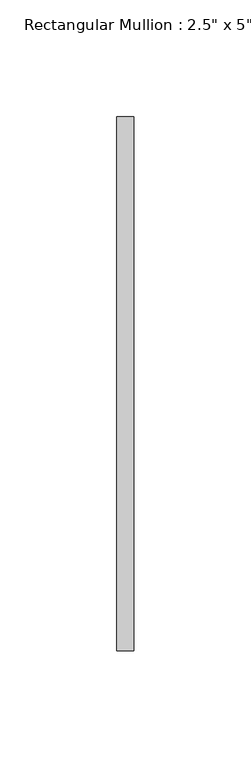
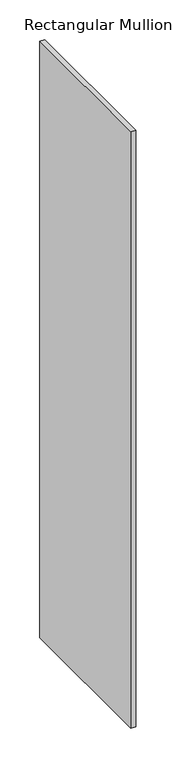
"""IFC4 building model written with IfcOpenShell, lengths in millimetres: member geometry."""

from ifc_helpers import new_model, si_unit, frame, origin, place, context, project, spatial, polyline, outline, extrude, source, transform, mapped, element, save


def member_065c0f10(model_context):
    return source(origin(), model_context, "Body", "SweptSolid", [
        extrude(outline(polyline([(0.0, 114.3), (0.0, -114.3), (-7.239, -114.3), (-7.239, 114.3), (0.0, 114.3)])), frame((0.0, 0.0, -914.4), z_axis=(0.0, 0.0, 1.0), x_axis=(1.0, 0.0, 0.0)), (0.0, 0.0, 1.0), 914.4),
    ])


if __name__ == "__main__":
    model = new_model("IFC4")
    model_context = context("Model", 3, world=origin())
    ifc_project = project(units=[si_unit("LENGTHUNIT", "METRE", prefix="MILLI")], contexts=[model_context])
    site = spatial("IfcSite", under=ifc_project)
    building = spatial("IfcBuilding", under=site)
    placement = place(None, origin())
    member_shape = member_065c0f10(model_context)
    element("IfcMember", 1, ObjectType="Rectangular Mullion : 2.5\" x 5\" rectangular", at=placement, inside=building, context=model_context, shape_type="MappedRepresentation", body=[
        mapped(member_shape, transform((0.0, 0.0, 0.0), x_axis=(1.0, 0.0, 0.0), y_axis=(0.0, 1.0, 0.0), z_axis=(0.0, 0.0, 1.0))),
    ])
    save(model, "model.ifc")

# Revit data of these elements
# Type "Rectangular Mullion : 2.5\" x 5\" rectangular"
#   built-in parameter 1007304 = 0.75 (stored number, unit not read)
#   built-in parameter 1007301 = 0.011875 (stored number, unit not read)
#   built-in parameter 1007300 = 0.011875 (stored number, unit not read)
# Element 1 (IfcMember, "Rectangular Mullion : 2.5\" x 5\" rectangular")
#   Materials on its faces: "WINDOW GLASS MATERIAL"
# Materials
#   "WINDOW GLASS MATERIAL": class "Generic", colour RGB 120 120 120, transparency 0, Cost = 0
